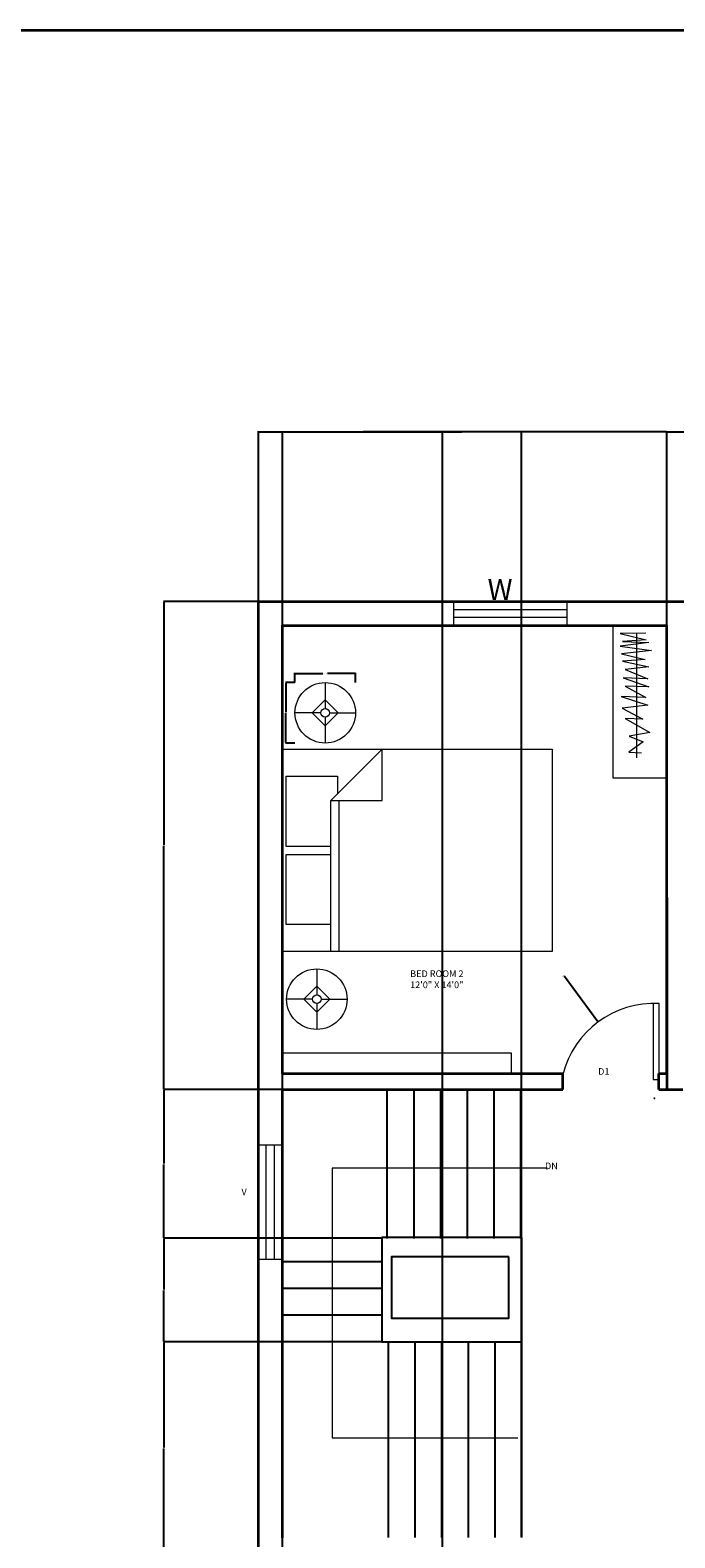
# Model space of a CAD drawing. Units: inches. Extents: x 65 to 1274, y 42 to 1041.
# Tile 5 of 6: x 678 to 920, y 476 to 1041. Entities that reach past the tile are written whole.
import ezdxf

# ---------------------------------------------------------------- set-up
doc = ezdxf.new("R2010")
doc.units = ezdxf.units.IN
for name, color, linetype, lineweight in [('A-ANNO-DIMS', 2, 'Continuous', 18), ('A-ANNO-SYMB', 7, 'Continuous', 13), ('A-AREA-IDEN', 7, 'Continuous', 18), ('A-DOOR', 3, 'Continuous', 18), ('A-FLOR-CASE', 8, 'Continuous', 18), ('A-FLOR-STRS', 2, 'Continuous', 25), ('A-FURN', 8, 'Continuous', 18), ('A-GLAZ', 4, 'Continuous', 18), ('A-WALL', 7, 'Continuous', 35), ('Text', 7, 'Continuous', 18), ('Title Block', 7, 'Continuous', 35)]:
    doc.layers.add(name, color=color, linetype=linetype, lineweight=lineweight)
doc.styles.get("Standard").update_dxf_attribs({"font": 'arial.ttf'})
doc.dimstyles.get("Standard").update_dxf_attribs({"dimtxt": 0.18, "dimasz": 0.18, "dimexe": 0.18, "dimexo": 0.0625, "dimgap": 0.09, "dimtad": 0, "dimtih": 1, "dimtoh": 1, "dimdec": 4, "dimzin": 0, "dimdsep": 46, "dimtxsty": 'Standard', "dimcen": 0.09, "dimadec": 0, "dimazin": 0, "dimtfac": 1, "dimtdec": 4, "dimtofl": 0, "dimtmove": 0, "dimatfit": 3, "dimfxl": 1, "dimtolj": 1, "dimtzin": 0, "dimarcsym": 0})

# ---------------------------------------------------------------- blocks, each defined once
blk = doc.blocks.new('Bed - Queen')
for p, q in [((0, -80.00003), (0, 0)), ((0, 0), (59.99999, 0)), ((59.99999, 0), (59.99999, -80.00003)), ((7.99999, -1.2), (28.79998, -1.2)), ((7.99999, -14.4), (7.99999, -1.2)), ((28.79998, -1.2), (28.79998, -14.4)), ((31.19999, -1.2), (51.99999, -1.2)), ((31.19999, -14.4), (31.19999, -1.2)), ((51.99999, -1.2), (51.99999, -16.4)), ((0, -14.4), (44.8, -14.4)), ((44.8, -16.8), (0, -16.8)), ((59.99999, -29.6), (44.8, -14.4)), ((44.8, -14.4), (44.8, -29.6)), ((51.99999, -16.4), (46.79936, -16.4)), ((44.8, -29.6), (59.99999, -29.6)), ((59.99999, -80.00003), (0, -80.00003))]:
    blk.add_line(p, q)
blk = doc.blocks.new('Lamp - Table')
for p, q in [((0, 7), (0, 1)), ((-1, 0), (-7, 0)), ((0, 3), (-3, 0)), ((-3, 0), (0, -3)), ((3, 0), (0, 3)), ((0, -3), (3, 0)), ((1, 0), (7, 0)), ((0, -1), (0, -7))]:
    blk.add_line(p, q)
for radius in [7, 1]:
    blk.add_circle((0, 0), radius)
blk = doc.blocks.new('WIN-43-DEEP-FRAME')
for p, q in [((9, 42.65), (0, 42.65)), ((0, 42.65), (0, 0)), ((3, 0), (3, 42.65)), ((6, 42.65), (6, 0)), ((9, 0), (9, 42.65)), ((0, 0), (9, 0))]:
    blk.add_line(p, q)
blk = doc.blocks.new('*D38')
at = {"layer": 'A-ANNO-DIMS', "color": 0, "lineweight": -2, "transparency": 16777216}
for p, q in [((777.5, 796.81), (777.5, 800.33)), ((777.68, 800.15), (787.94, 800.15)), ((800, 800.15), (789.74, 800.15)), ((800.18, 796.81), (800.18, 800.33))]:
    blk.add_line(p, q, dxfattribs=at)
at = {"layer": 'A-ANNO-DIMS', "color": 0, "transparency": 16777216}
for points in [[(777.68, 800.18), (777.68, 800.12), (777.5, 800.15)], [(800, 800.18), (800, 800.12), (800.18, 800.15)]]:
    blk.add_solid(points, dxfattribs=at)
at = {"layer": 'Defpoints', "color": 0, "transparency": 16777216}
for p in [(800.18, 800.15), (777.5, 796.75), (800.18, 796.75)]:
    blk.add_point(p, dxfattribs=at)
at = {"layer": 'A-ANNO-DIMS', "color": 0, "transparency": 16777216, "insert": (788.84, 800.15), "char_height": 0.18, "attachment_point": 5}
blk.add_mtext('\\A1;LAMP 23 TYP.', dxfattribs=at)
blk = doc.blocks.new('*D39')
at = {"layer": 'A-ANNO-DIMS', "color": 0, "lineweight": -2, "transparency": 16777216}
for p, q in [((777.44, 796.75), (773.92, 796.75)), ((774.1, 796.57), (774.1, 785.59)), ((774.1, 774.25), (774.1, 785.23)), ((777.44, 774.07), (773.92, 774.07))]:
    blk.add_line(p, q, dxfattribs=at)
at = {"layer": 'A-ANNO-DIMS', "color": 0, "transparency": 16777216}
for points in [[(774.07, 796.57), (774.13, 796.57), (774.1, 796.75)], [(774.07, 774.25), (774.13, 774.25), (774.1, 774.07)]]:
    blk.add_solid(points, dxfattribs=at)
at = {"layer": 'Defpoints', "color": 0, "transparency": 16777216}
for p in [(774.1, 796.75), (777.5, 796.75), (777.5, 774.07)]:
    blk.add_point(p, dxfattribs=at)
at = {"layer": 'A-ANNO-DIMS', "color": 0, "transparency": 16777216, "insert": (774.1, 785.41), "char_height": 0.18, "attachment_point": 5}
blk.add_mtext('\\A1;23 TYP.', dxfattribs=at)
blk = doc.blocks.new('*D66')
at = {"layer": 'A-ANNO-DIMS', "color": 0, "lineweight": -2, "transparency": 16777216}
for p, q in [((763.83, 827.21), (763.83, 890.96)), ((764.01, 890.78), (840.05, 890.78)), ((916.65, 890.78), (840.61, 890.78)), ((916.83, 818.21), (916.83, 890.96))]:
    blk.add_line(p, q, dxfattribs=at)
at = {"layer": 'A-ANNO-DIMS', "color": 0, "transparency": 16777216}
for points in [[(764.01, 890.81), (764.01, 890.75), (763.83, 890.78)], [(916.65, 890.81), (916.65, 890.75), (916.83, 890.78)]]:
    blk.add_solid(points, dxfattribs=at)
at = {"layer": 'Defpoints', "color": 0, "transparency": 16777216}
for p in [(916.83, 890.78), (763.83, 827.15), (916.83, 818.15)]:
    blk.add_point(p, dxfattribs=at)
at = {"layer": 'A-ANNO-DIMS', "color": 0, "transparency": 16777216, "insert": (840.33, 890.78), "char_height": 0.18, "attachment_point": 5}
blk.add_mtext('\\A1;153', dxfattribs=at)
blk = doc.blocks.new('*D67')
at = {"layer": 'A-ANNO-DIMS', "color": 0, "lineweight": -2, "transparency": 16777216}
for p, q in [((916.83, 818.21), (916.83, 890.96)), ((917.01, 890.78), (1032.06, 890.78)), ((1147.65, 890.78), (1032.6, 890.78)), ((1147.83, 827.21), (1147.83, 890.96))]:
    blk.add_line(p, q, dxfattribs=at)
at = {"layer": 'A-ANNO-DIMS', "color": 0, "transparency": 16777216}
for points in [[(917.01, 890.81), (917.01, 890.75), (916.83, 890.78)], [(1147.65, 890.81), (1147.65, 890.75), (1147.83, 890.78)]]:
    blk.add_solid(points, dxfattribs=at)
at = {"layer": 'Defpoints', "color": 0, "transparency": 16777216}
for p in [(1147.83, 890.78), (1147.83, 827.15), (916.83, 818.15)]:
    blk.add_point(p, dxfattribs=at)
at = {"layer": 'A-ANNO-DIMS', "color": 0, "transparency": 16777216, "insert": (1032.33, 890.78), "char_height": 0.18, "attachment_point": 5}
blk.add_mtext('\\A1;231', dxfattribs=at)
blk = doc.blocks.new('*D73')
at = {"layer": 'A-ANNO-DIMS', "color": 0, "lineweight": -2, "transparency": 16777216}
for p, q in [((772.48, 549.58), (728.22, 549.58)), ((728.4, 549.4), (728.4, 510.05)), ((728.4, 470.33), (728.4, 509.68)), ((772.77, 470.15), (728.22, 470.15))]:
    blk.add_line(p, q, dxfattribs=at)
at = {"layer": 'A-ANNO-DIMS', "color": 0, "transparency": 16777216}
for points in [[(728.37, 549.4), (728.43, 549.4), (728.4, 549.58)], [(728.37, 470.33), (728.43, 470.33), (728.4, 470.15)]]:
    blk.add_solid(points, dxfattribs=at)
at = {"layer": 'Defpoints', "color": 0, "transparency": 16777216}
for p in [(728.4, 549.58), (772.55, 549.58), (772.83, 470.15)]:
    blk.add_point(p, dxfattribs=at)
at = {"layer": 'A-ANNO-DIMS', "color": 0, "transparency": 16777216, "insert": (728.4, 509.86), "char_height": 0.18, "attachment_point": 5}
blk.add_mtext('\\A1;79.43', dxfattribs=at)
blk = doc.blocks.new('*D74')
at = {"layer": 'A-ANNO-DIMS', "color": 0, "lineweight": -2, "transparency": 16777216}
for p, q in [((772.8, 588.47), (728.22, 588.47)), ((728.4, 588.29), (728.4, 569.21)), ((728.4, 549.76), (728.4, 568.85)), ((772.48, 549.58), (728.22, 549.58))]:
    blk.add_line(p, q, dxfattribs=at)
at = {"layer": 'A-ANNO-DIMS', "color": 0, "transparency": 16777216}
for points in [[(728.37, 588.29), (728.43, 588.29), (728.4, 588.47)], [(728.37, 549.76), (728.43, 549.76), (728.4, 549.58)]]:
    blk.add_solid(points, dxfattribs=at)
at = {"layer": 'Defpoints', "color": 0, "transparency": 16777216}
for p in [(728.4, 588.47), (772.86, 588.47), (772.55, 549.58)]:
    blk.add_point(p, dxfattribs=at)
at = {"layer": 'A-ANNO-DIMS', "color": 0, "transparency": 16777216, "insert": (728.4, 569.03), "char_height": 0.18, "attachment_point": 5}
blk.add_mtext('\\A1;38.89', dxfattribs=at)
blk = doc.blocks.new('*D75')
at = {"layer": 'A-ANNO-DIMS', "color": 0, "lineweight": -2, "transparency": 16777216}
for p, q in [((772.77, 644.15), (728.22, 644.15)), ((728.4, 643.97), (728.4, 616.49)), ((728.4, 588.65), (728.4, 616.13)), ((772.8, 588.47), (728.22, 588.47))]:
    blk.add_line(p, q, dxfattribs=at)
at = {"layer": 'A-ANNO-DIMS', "color": 0, "transparency": 16777216}
for points in [[(728.37, 643.97), (728.43, 643.97), (728.4, 644.15)], [(728.37, 588.65), (728.43, 588.65), (728.4, 588.47)]]:
    blk.add_solid(points, dxfattribs=at)
at = {"layer": 'Defpoints', "color": 0, "transparency": 16777216}
for p in [(728.4, 644.15), (772.83, 644.15), (772.86, 588.47)]:
    blk.add_point(p, dxfattribs=at)
at = {"layer": 'A-ANNO-DIMS', "color": 0, "transparency": 16777216, "insert": (728.4, 616.31), "char_height": 0.18, "attachment_point": 5}
blk.add_mtext('\\A1;55.67', dxfattribs=at)
blk = doc.blocks.new('*D76')
at = {"layer": 'A-ANNO-DIMS', "color": 0, "lineweight": -2, "transparency": 16777216}
for p, q in [((763.77, 827.15), (728.22, 827.15)), ((728.4, 826.97), (728.4, 735.83)), ((728.4, 644.33), (728.4, 735.47)), ((772.77, 644.15), (728.22, 644.15))]:
    blk.add_line(p, q, dxfattribs=at)
at = {"layer": 'A-ANNO-DIMS', "color": 0, "transparency": 16777216}
for points in [[(728.37, 826.97), (728.43, 826.97), (728.4, 827.15)], [(728.37, 644.33), (728.43, 644.33), (728.4, 644.15)]]:
    blk.add_solid(points, dxfattribs=at)
at = {"layer": 'Defpoints', "color": 0, "transparency": 16777216}
for p in [(728.4, 827.15), (763.83, 827.15), (772.83, 644.15)]:
    blk.add_point(p, dxfattribs=at)
at = {"layer": 'A-ANNO-DIMS', "color": 0, "transparency": 16777216, "insert": (728.4, 735.65), "char_height": 0.18, "attachment_point": 5}
blk.add_mtext('\\A1;183', dxfattribs=at)
blk = doc.blocks.new('*D77')
at = {"layer": 'A-ANNO-DIMS', "color": 0, "lineweight": -2, "transparency": 16777216}
for p, q in [((772.83, 374.21), (772.83, 890.96)), ((773.01, 890.78), (802.61, 890.78)), ((832.65, 890.78), (803.05, 890.78)), ((832.83, 374.21), (832.83, 890.96))]:
    blk.add_line(p, q, dxfattribs=at)
at = {"layer": 'A-ANNO-DIMS', "color": 0, "transparency": 16777216}
for points in [[(773.01, 890.81), (773.01, 890.75), (772.83, 890.78)], [(832.65, 890.81), (832.65, 890.75), (832.83, 890.78)]]:
    blk.add_solid(points, dxfattribs=at)
at = {"layer": 'Defpoints', "color": 0, "transparency": 16777216}
for p in [(832.83, 890.78), (772.83, 374.15), (832.83, 374.15)]:
    blk.add_point(p, dxfattribs=at)
at = {"layer": 'A-ANNO-DIMS', "color": 0, "transparency": 16777216, "insert": (802.83, 890.78), "char_height": 0.18, "attachment_point": 5}
blk.add_mtext('\\A1;60', dxfattribs=at)
blk = doc.blocks.new('*D78')
at = {"layer": 'A-ANNO-DIMS', "color": 0, "lineweight": -2, "transparency": 16777216}
for p, q in [((772.83, 476.21), (772.83, 890.96)), ((773.01, 890.78), (817.21, 890.78)), ((862.2, 890.78), (818, 890.78)), ((862.38, 476.39), (862.38, 890.96))]:
    blk.add_line(p, q, dxfattribs=at)
at = {"layer": 'A-ANNO-DIMS', "color": 0, "transparency": 16777216}
for points in [[(773.01, 890.81), (773.01, 890.75), (772.83, 890.78)], [(862.2, 890.81), (862.2, 890.75), (862.38, 890.78)]]:
    blk.add_solid(points, dxfattribs=at)
at = {"layer": 'Defpoints', "color": 0, "transparency": 16777216}
for p in [(862.38, 890.78), (772.83, 476.15), (862.38, 476.33)]:
    blk.add_point(p, dxfattribs=at)
at = {"layer": 'A-ANNO-DIMS', "color": 0, "transparency": 16777216, "insert": (817.6, 890.78), "char_height": 0.18, "attachment_point": 5}
blk.add_mtext('\\A1;89.55', dxfattribs=at)
blk = doc.blocks.new('*D81')
at = {"layer": 'A-ANNO-DIMS', "color": 0, "lineweight": -2, "transparency": 16777216}
for p, q in [((878.28, 686.67), (878.46, 686.67)), ((878.46, 686.67), (891.01, 669.68)), ((912.12, 640.98), (912.3, 640.98)), ((912.21, 640.89), (912.21, 641.07))]:
    blk.add_line(p, q, dxfattribs=at)
at = {"layer": 'A-ANNO-DIMS', "color": 0, "transparency": 16777216}
blk.add_solid([(891.04, 669.7), (890.99, 669.66), (891.12, 669.54)], dxfattribs=at)
at = {"layer": 'Defpoints', "color": 0, "transparency": 16777216}
for p in [(891.12, 669.54), (912.21, 640.98)]:
    blk.add_point(p, dxfattribs=at)
at = {"layer": 'A-ANNO-DIMS', "color": 0, "transparency": 16777216, "insert": (877.73, 686.67), "char_height": 0.18, "attachment_point": 5}
blk.add_mtext('\\A1;R35.504', dxfattribs=at)

msp = doc.modelspace()

# ---------------------------------------------------------------- linework, layer by layer
at = {"layer": 'A-ANNO-SYMB'}
for p, q in [((871.9738, 614.7315), (791.4502, 614.7315)), ((791.4502, 614.7315), (791.4502, 513.6346)), ((791.4502, 513.6346), (861.0485, 513.6346))]:
    msp.add_line(p, q, dxfattribs=at)
at = {"layer": 'A-DOOR'}
msp.add_lwpolyline([(913.9698, 676.4909), (911.7125, 676.4909), (911.7125, 647.9693), (913.9698, 647.9693)], close=True, dxfattribs=at)
msp.add_arc((912.2106, 640.9782), 35.5044, 87.202264, 165.693589, dxfattribs=at)
at = {"layer": 'A-FLOR-CASE'}
for p, q in [((896.7128, 760.9233), (896.7128, 817.8088)), ((909.0167, 815.3046), (899.3342, 815.1203)), ((899.3342, 815.1203), (909.1089, 812.7242)), ((905.4203, 815.3046), (905.4203, 768.4893)), ((910.1232, 811.7105), (899.3342, 810.3282)), ((899.3342, 810.3282), (911.0453, 808.7615)), ((911.0453, 808.7615), (899.7953, 807.5635)), ((909.1089, 812.7242), (900.1641, 812.0791)), ((900.1641, 812.0791), (910.1232, 811.7105)), ((899.7953, 807.5635), (908.74, 805.3517)), ((908.74, 805.3517), (900.1641, 804.7988)), ((900.1641, 804.7988), (910.031, 802.6792)), ((910.031, 802.6792), (901.2707, 801.5734)), ((909.6621, 798.1636), (900.4408, 798.5322)), ((900.4408, 798.5322), (910.1232, 795.1224)), ((901.2707, 801.5734), (909.6621, 798.1636)), ((908.9244, 791.1597), (899.7031, 791.5283)), ((899.7031, 791.5283), (909.6621, 788.3029)), ((910.1232, 795.1224), (901.1785, 795.3989)), ((901.1785, 795.3989), (908.9244, 791.1597)), ((909.6621, 788.3029), (900.0719, 787.197)), ((900.0719, 787.197), (907.8179, 782.9578)), ((907.8179, 782.9578), (901.2707, 783.2343)), ((901.2707, 783.2343), (910.3999, 778.0736)), ((907.9101, 774.5716), (902.6539, 770.7011)), ((910.3999, 778.0736), (902.7461, 776.6912)), ((902.7461, 776.6912), (907.9101, 774.5716)), ((902.6539, 770.7011), (907.3568, 770.4246)), ((916.941, 760.9233), (896.7128, 760.9233)), ((858.6045, 657.7852), (772.9938, 657.7852)), ((858.6045, 650.0073), (858.6045, 657.7852))]:
    msp.add_line(p, q, dxfattribs=at)
at = {"layer": 'A-FLOR-STRS'}
for p, q in [((812.1072, 588.3428), (812.1072, 644.2496)), ((822.1072, 588.3428), (822.1072, 644.2496)), ((832.1072, 588.3428), (832.1072, 644.2496)), ((842.1072, 588.3428), (842.1072, 644.2496)), ((852.1072, 588.3428), (852.1072, 644.2496)), ((862.1072, 588.3428), (862.1072, 644.2496)), ((809.8807, 588.4738), (772.8621, 588.4738)), ((810.0389, 579.5812), (772.5457, 579.5812)), ((810.0389, 569.5812), (772.5457, 569.5812)), ((810.0389, 559.5812), (772.5457, 559.5812)), ((810.0389, 549.5812), (772.5457, 549.5812)), ((812.3772, 549.5222), (812.3772, 476.3306)), ((822.3772, 549.5222), (822.3772, 476.3306)), ((832.3772, 549.5222), (832.3772, 476.3306)), ((842.3772, 549.5222), (842.3772, 476.3306)), ((852.3772, 549.5222), (852.3772, 476.3306)), ((862.3772, 549.5222), (862.3772, 476.3306))]:
    msp.add_line(p, q, dxfattribs=at)
for points in [[(862.4642, 588.714), (810.0547, 588.714), (810.0547, 549.633), (862.4642, 549.633)], [(857.6287, 581.4429), (813.6854, 581.4429), (813.6854, 558.4778), (857.6287, 558.4778)]]:
    msp.add_lwpolyline(points, close=True, dxfattribs=at)
at = {"layer": 'A-WALL'}
for p, q in [((763.8297, 284.1476), (763.8297, 827.1476)), ((763.8297, 827.1476), (1147.8298, 827.1476)), ((772.8297, 818.1476), (916.8297, 818.1476)), ((772.8297, 650.1476), (772.8297, 818.1476)), ((916.8297, 650.1476), (916.8297, 818.1476)), ((916.8297, 716.1476), (916.8297, 644.1476)), ((772.8297, 650.1476), (877.8298, 650.1476)), ((877.8298, 644.1476), (877.8298, 650.1476)), ((913.8298, 644.1476), (913.8298, 650.1476)), ((913.8298, 650.1476), (916.8297, 650.1476)), ((772.8297, 644.1476), (877.8298, 644.1476)), ((772.8297, 476.1476), (772.8297, 644.1476)), ((913.8298, 644.1476), (922.8298, 644.1476))]:
    msp.add_line(p, q, dxfattribs=at)
at = {"layer": 'Title Block'}
msp.add_lwpolyline([(64.7421, 1041.286), (1273.976, 1041.286), (1273.976, 41.6396), (64.7421, 41.6396)], close=True, dxfattribs=at)

# ---------------------------------------------------------------- block references
at = {"layer": 'A-FURN', "xscale": 1.619462315136964, "yscale": 1.619462315136964, "zscale": 1.619462315136964}
for p in [(788.8412, 785.409), (785.6822, 678.0709)]:
    msp.add_blockref('Lamp - Table', p, dxfattribs=at)
at = {"layer": 'A-FURN', "xscale": 1.264723082454659, "yscale": 1.264723082454659, "zscale": 1.264723082454659, "rotation": 89.99999999999999}
msp.add_blockref('Bed - Queen', (772.7322, 695.878), dxfattribs=at)
at = {"layer": 'A-GLAZ'}
for p, rotation in [((836.8919, 827.136), 270), ((772.6555, 623.3044), 180)]:
    msp.add_blockref('WIN-43-DEEP-FRAME', p, dxfattribs=dict(at, rotation=rotation))

# ---------------------------------------------------------------- texts
at = {"layer": 'A-AREA-IDEN', "insert": (820.6523, 688.8597), "char_height": 2.5, "attachment_point": 1}
msp.add_mtext_dynamic_manual_height_columns('BED ROOM 2\\P12\'0" X 14\'0"', width=42.877242, gutter_width=12.5, heights=[0], dxfattribs=at)
at = {"layer": 'Text', "attachment_point": 1}
for s, width, gutter_width, insert, char_height in [('W', 96.254197, 39.1027, (849.6634, 835.5506), 7.8205), ('D1', 23.109077, 12.5, (891.0899, 652.206), 2.5), ('DN', 4.674936, 12.5, (871.1704, 616.8132), 2.5), ('V', 5.099062, 12.5, (757.4585, 607.082), 2.5)]:
    msp.add_mtext_dynamic_manual_height_columns(s, width=width, gutter_width=gutter_width, heights=[0], dxfattribs=dict(at, insert=insert, char_height=char_height))

# ---------------------------------------------------------------- dimensions: what is measured, and where the dimension line sits
at = {"layer": 'A-ANNO-DIMS'}
for base, p1, p2, override, picture, middle in [((916.8297, 890.7807), (763.8297, 827.1476), (916.8297, 818.1476), {"dimdec": 0, "dimlfac": 1, "dimrnd": 0, "dimzin": 0, "dimdsep": 46, "dimlunit": 2}, '*D66', (840.3297, 890.7807)), ((832.8297, 890.7807), (772.8297, 374.1476), (832.8297, 374.1476), {"dimdec": 0, "dimlfac": 1, "dimrnd": 0, "dimzin": 0, "dimdsep": 46, "dimlunit": 2}, '*D77', (802.8297, 890.7807)), ((862.3772, 890.7807), (772.8297, 476.1476), (862.3772, 476.3306), {"dimdec": 2, "dimlfac": 1, "dimrnd": 0, "dimzin": 0, "dimdsep": 46, "dimlunit": 2}, '*D78', (817.6035, 890.7807)), ((1147.8298, 890.7807), (916.8297, 818.1476), (1147.8298, 827.1476), {"dimdec": 0, "dimlfac": 1, "dimrnd": 0, "dimzin": 0, "dimdsep": 46, "dimlunit": 2}, '*D67', (1032.3298, 890.7807))]:
    dim = msp.add_linear_dim(base=base, p1=p1, p2=p2, dimstyle='Standard', override=override, dxfattribs=at)
    dim.commit()
    dim.dimension.update_dxf_attribs({"geometry": picture, "text_midpoint": middle})
for base, p1, p2, override, picture, middle in [((728.4012, 827.1476), (772.8297, 644.1476), (763.8297, 827.1476), {"dimdec": 0, "dimlfac": 1, "dimrnd": 0, "dimzin": 0, "dimdsep": 46, "dimlunit": 2}, '*D76', (728.4012, 735.6476)), ((728.4012, 644.1476), (772.8621, 588.4738), (772.8297, 644.1476), {"dimdec": 2, "dimlfac": 1, "dimrnd": 0, "dimzin": 0, "dimdsep": 46, "dimlunit": 2}, '*D75', (728.4012, 616.3107)), ((728.4012, 588.4738), (772.5457, 549.5812), (772.8621, 588.4738), {"dimdec": 2, "dimlfac": 1, "dimrnd": 0, "dimzin": 0, "dimdsep": 46, "dimlunit": 2}, '*D74', (728.4012, 569.0275)), ((728.4012, 549.5812), (772.8297, 470.1476), (772.5457, 549.5812), {"dimdec": 2, "dimlfac": 1, "dimrnd": 0, "dimzin": 0, "dimdsep": 46, "dimlunit": 2}, '*D73', (728.4012, 509.8644))]:
    dim = msp.add_linear_dim(base=base, p1=p1, p2=p2, angle=90, dimstyle='Standard', override=override, dxfattribs=at)
    dim.commit()
    dim.dimension.update_dxf_attribs({"geometry": picture, "text_midpoint": middle})
dim = msp.add_linear_dim(base=(800.1774, 800.1461), p1=(777.505, 796.7452), p2=(800.1774, 796.7452), text='LAMP <> TYP.', dimstyle='Standard', override={"dimdec": 0, "dimlfac": 1, "dimrnd": 0, "dimzin": 0, "dimdsep": 46, "dimlunit": 2}, dxfattribs=at)
dim.commit()
dim.dimension.update_dxf_attribs({"geometry": '*D38', "text_midpoint": (788.8412, 800.1461)})
dim = msp.add_linear_dim(base=(774.1041, 796.7452), p1=(777.505, 774.0728), p2=(777.505, 796.7452), angle=90, text='<> TYP.', dimstyle='Standard', override={"dimdec": 0, "dimlfac": 1, "dimrnd": 0, "dimzin": 0, "dimdsep": 46, "dimlunit": 2}, dxfattribs=at)
dim.commit()
dim.dimension.update_dxf_attribs({"geometry": '*D39', "text_midpoint": (774.1041, 785.409)})
dim = msp.add_radius_dim(center=(912.2106, 640.9782), mpoint=(891.118, 669.538), dimstyle='Standard', override={"dimdec": 3, "dimlfac": 1, "dimrnd": 0, "dimzin": 0, "dimdsep": 46, "dimlunit": 2}, dxfattribs=at)
dim.commit()
dim.dimension.update_dxf_attribs({"geometry": '*D81', "text_midpoint": (877.733, 686.6739), "dimtype": 164})

doc.saveas('drawing.dxf')
